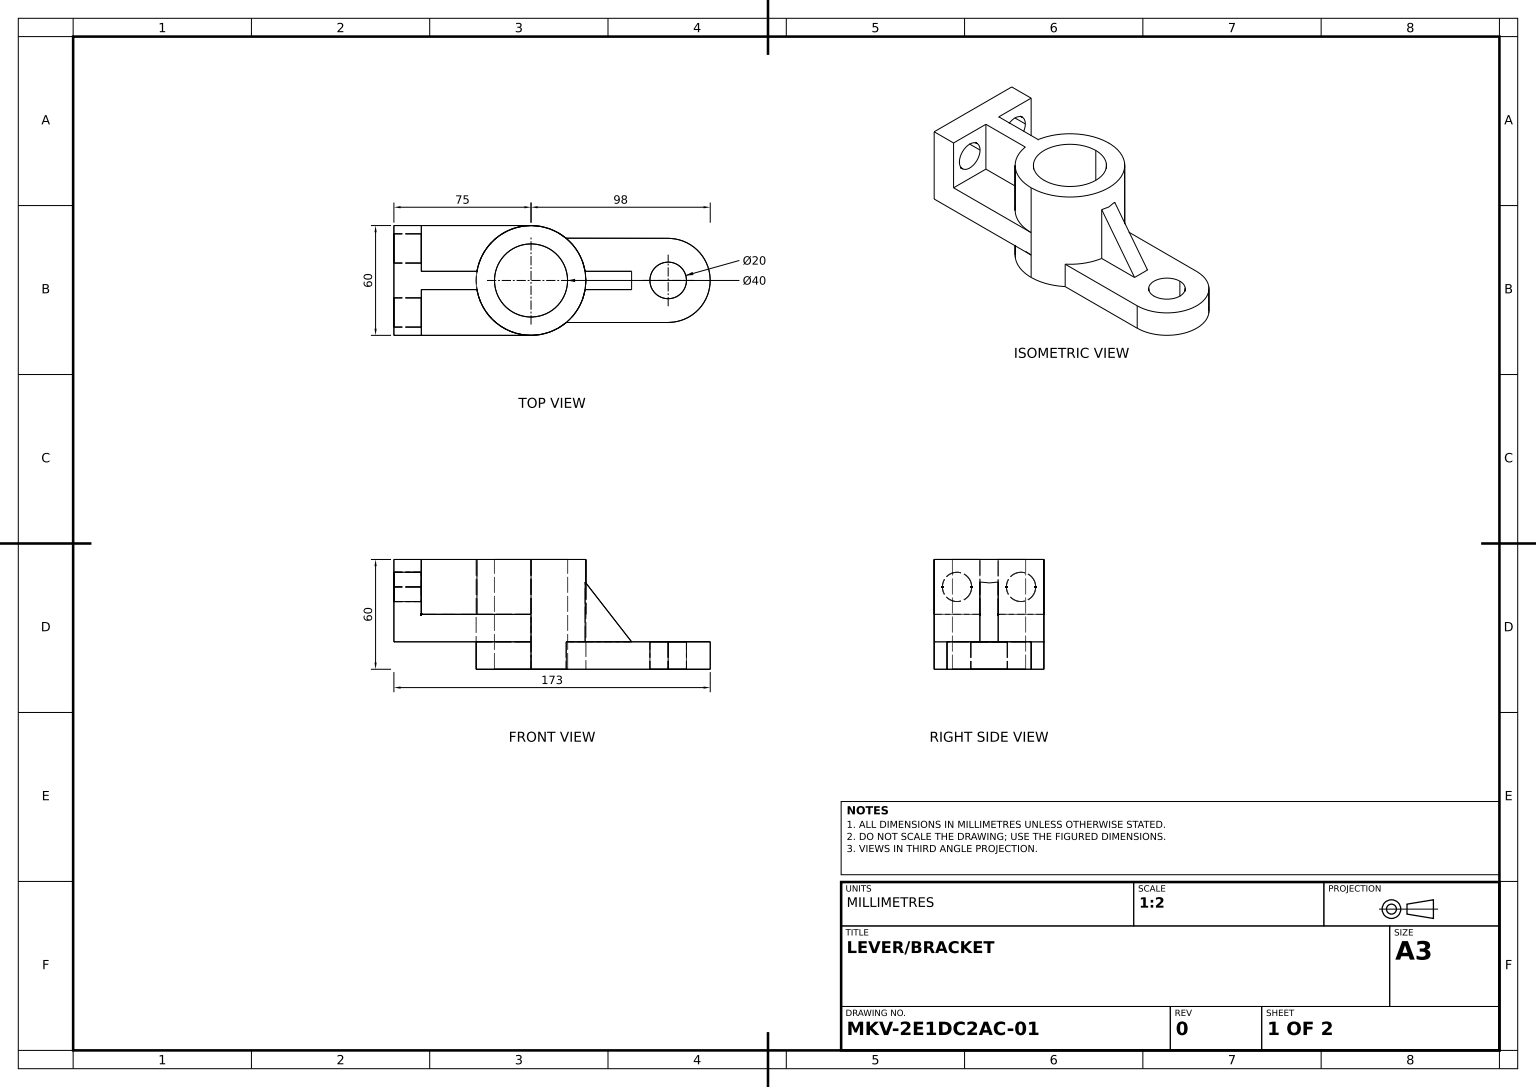
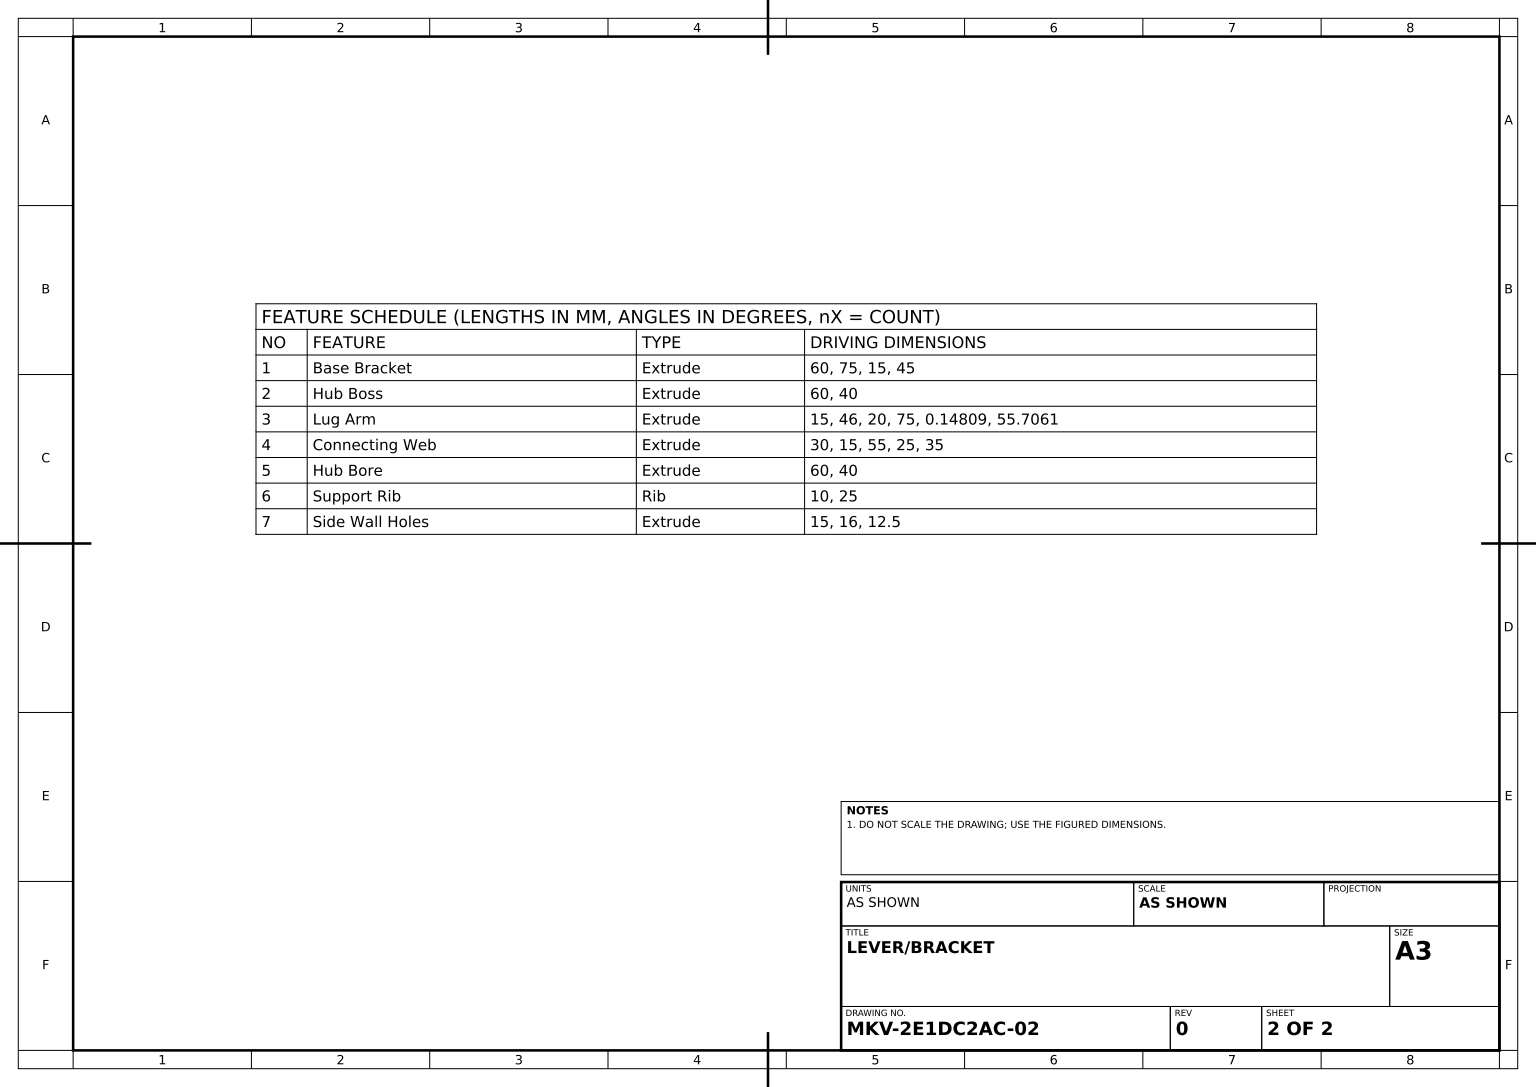
SolidWorks part; units mm, degrees
material "Plain Carbon Steel"
ref_plane "Front Plane" through (0, 0, 0) normal (0, 0, 1) x (1, 0, 0)
ref_plane "Top Plane" through (0, 0, 0) normal (0, 1, 0) x (1, 0, 0)
ref_plane "Right Plane" through (0, 0, 0) normal (1, 0, 0) x (0, 0, -1)
sketch "Base Bracket Profile Sketch" plane through (0, 0, 0) normal (0, 0, 1) x (1, 0, 0)
  line L1 (0, 15) -> (-75, 15)
  line L2 (-75, 15) -> (-75, 60)
  line L3 (-75, 60) -> (-60, 60)
  line L4 (-60, 60) -> (-60, 30)
  line L5 (-60, 30) -> (0, 30)
  line L6 (0, 30) -> (0, 15)
  dimension "D1" = 75
  dimension "D2" = 15
  dimension "D3" = 45
  dimension "D4" = 15
  dimension "D5" = 60
  dimension "D6" = 15
extrude "Base Bracket" add sketch "Base Bracket Profile Sketch" along normal mid plane 60
sketch "Hub Boss Sketch" plane through (0, 0, 0) normal (0, 1, 0) x (1, 0, 0)
  circle A2 centre (0, 0) radius 30
  circle A3 centre (0, 0) radius 20
  dimension "D1" = 40
  dimension "D2" = 60
extrude "Hub Boss" add sketch "Hub Boss Sketch" along normal blind 60
sketch "Lug Arm Sketch" plane through (0, 0, 0) normal (0, 1, 0) x (1, 0, 0)
  line L0 (75, 23.0273) -> (19.1458, 23.0963)
  line L1 (19.1458, 23.0963) -> (19.2939, 5.2674)
  line L2 (19.2939, -5.2674) -> (19.2939, -22.9727)
  line L3 (19.2939, -22.9727) -> (75, -22.9727)
  line L4 (0, 0) -> (75, 0.0273) construction
  arc A0 (75, -22.9727) -> (75, 23.0273) centre (75, 0.0273) ccw
  circle A1 centre (75, 0.0273) radius 10
  circle A2 centre (0, 0) radius 30 construction
  circle A3 centre (0, 0) radius 20 construction
  arc A4 (19.2939, -5.2674) -> (19.2939, 5.2674) centre (0, 0) ccw
  dimension "D1" = 46
  dimension "D2" = 20
  dimension "D3" = 75
  dimension "D4" = 55.7061
  dimension "D5" = 0.1481
extrude "Lug Arm" add sketch "Lug Arm Sketch" along normal blind 15
sketch "Connecting Web Sketch" plane through (0, 60, 0) normal (0, 1, 0) x (1, 0, 0)
  line L0 (-75, -30) -> (-75, 30) construction
  line L1 (-60, 30) -> (-75, 30) construction
  line L2 (-60, -5) -> (-20, -5)
  line L3 (-60, 5) -> (-20, 5)
  line L4 (-60, 5) -> (-60, -5)
  line L5 (-20, 5) -> (-20, -5)
  dimension "D1" = 15
  dimension "D2" = 55
  dimension "D3" = 25
  dimension "D4" = 35
extrude "Connecting Web" add sketch "Connecting Web Sketch" against normal blind 30
sketch "Hub Bore Sketch" plane through (0, 60, 0) normal (0, 1, 0) x (1, 0, 0)
  circle A0 centre (0, 0) radius 20
  dimension "D1" = 40
extrude "Hub Bore" cut sketch "Hub Bore Sketch" against normal blind 60
sketch "Support Rib Sketch" plane through (0, 0, 0) normal (0, 0, 1) x (1, 0, 0)
  line L0 (20, 60) -> (55, 15)
  line L1 (19.2939, 15) -> (75, 15) construction
  dimension "D1" = 25
rib "Support Rib" sketch "Support Rib Sketch" sketch "Support Rib Sketch" thickness 10 extrusion direction parallel to sketch draft on no parameters "D1"=10
sketch "Side Wall Holes Sketch" plane through (-75, 0, 0) normal (-1, 0, 0) x (0, 0, 1)
  line L0 (30, 60) -> (-30, 60) construction
  line L1 (-30, 60) -> (-30, 15) construction
  line L2 (30, 60) -> (30, 15) construction
  circle A0 centre (-17.5, 45) radius 8
  circle A1 centre (17.5, 45) radius 8
  dimension "D3" = 16
  dimension "D4" = 16
  dimension "D1" = 15
  dimension "D2" = 15
  dimension "D5" = 12.5
  dimension "D6" = 12.5
  dimension "D7" = 35
extrude "Side Wall Holes" cut sketch "Side Wall Holes Sketch" against normal blind 15
